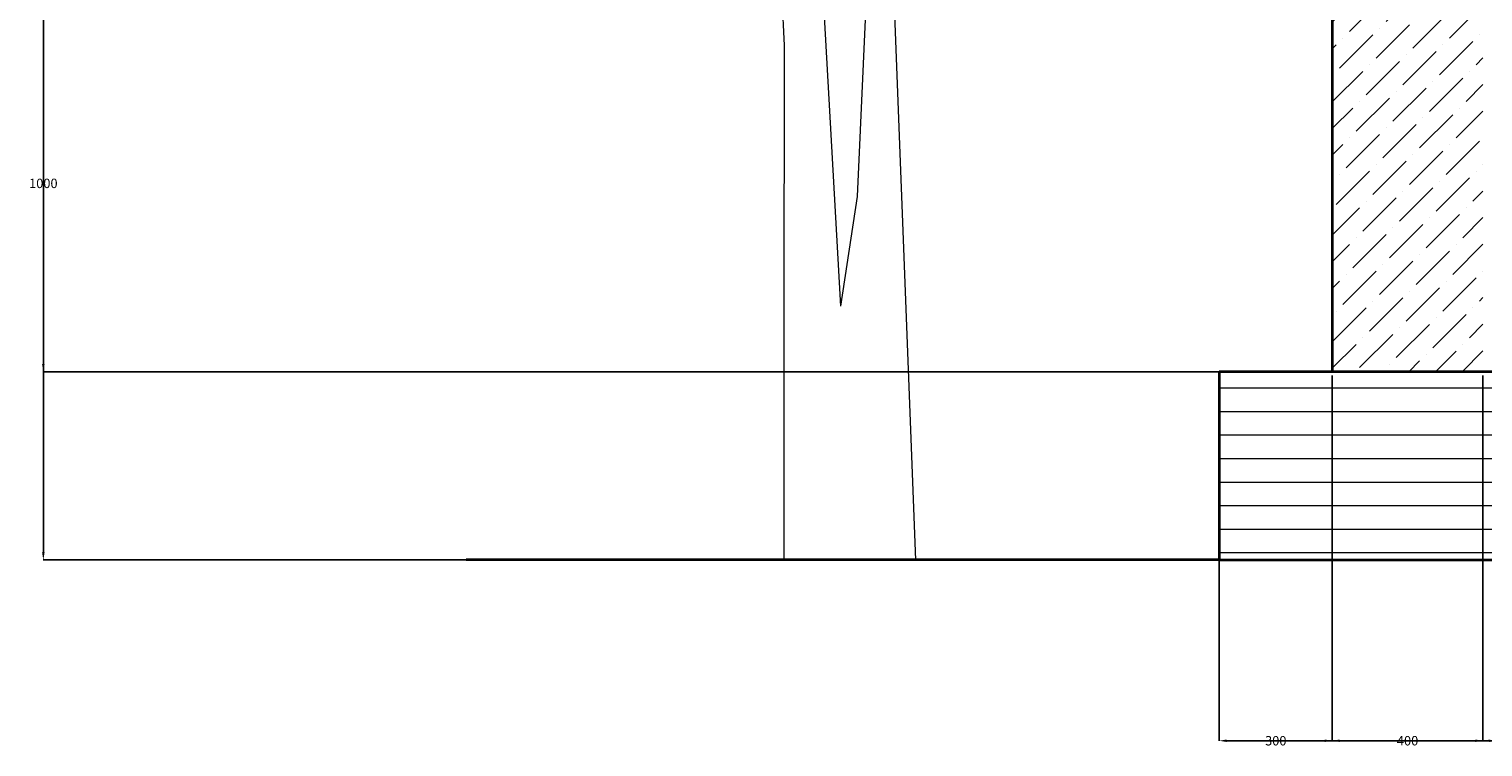
# Model space of a CAD drawing. Units: millimetres. Extents: x -692 to 9639, y -141 to 10345.
# Tile 1 of 19: x -687 to 3174, y -141 to 1765. Entities that reach past the tile are written whole.
import ezdxf

# ---------------------------------------------------------------- set-up
doc = ezdxf.new("R2010")
doc.units = ezdxf.units.MM
doc.header["$MEASUREMENT"] = 0
for name, color, linetype, lineweight in [('A-ANNO-DIMS', 2, 'Continuous', 18), ('A-ELEV', 7, 'Continuous', 35), ('A-ELEV-PATT', 8, 'Continuous', 13), ('L-PLNT', 3, 'Continuous', 18)]:
    doc.layers.add(name, color=color, linetype=linetype, lineweight=lineweight)
doc.styles.get("Standard").update_dxf_attribs({"font": 'arial.ttf'})
doc.dimstyles.get("Standard").update_dxf_attribs({"dimtxt": 25, "dimasz": 20, "dimexe": 0.18, "dimexo": 10, "dimgap": 10, "dimtad": 0, "dimtih": 1, "dimtoh": 1, "dimdec": 0, "dimzin": 0, "dimdsep": 46, "dimtxsty": 'Standard', "dimcen": 10, "dimadec": 0, "dimazin": 0, "dimtfac": 1, "dimtdec": 0, "dimtofl": 0, "dimtmove": 0, "dimatfit": 3, "dimfxl": 1, "dimtolj": 1, "dimtzin": 0, "dimarcsym": 0})

# ---------------------------------------------------------------- blocks, each defined once
blk = doc.blocks.new('*D6')
at = {"layer": 'A-ANNO-DIMS', "color": 0, "lineweight": -2, "transparency": 16777216}
for p, q in [((2473.7, 345.6), (2473.7, -124.6)), ((9073.7, 345.6), (9073.7, -124.6)), ((2493.7, -124.4), (5726.4, -124.4)), ((9053.7, -124.4), (5821.1, -124.4))]:
    blk.add_line(p, q, dxfattribs=at)
at = {"layer": 'A-ANNO-DIMS', "color": 0, "lineweight": -3, "transparency": 16777216}
for points in [[(2493.7, -121.1), (2493.7, -127.8), (2473.7, -124.4)], [(9053.7, -121.1), (9053.7, -127.8), (9073.7, -124.4)]]:
    blk.add_solid(points, dxfattribs=at)
at = {"layer": 'Defpoints', "color": 0, "lineweight": -3, "transparency": 16777216}
for p in [(2473.7, 355.6), (9073.7, 355.6), (9073.7, -124.4)]:
    blk.add_point(p, dxfattribs=at)
at = {"layer": 'A-ANNO-DIMS', "color": 0, "transparency": 16777216, "insert": (5773.7, -124.4), "char_height": 25, "attachment_point": 5}
blk.add_mtext('\\A1;6600', dxfattribs=at)
blk = doc.blocks.new('*D7')
at = {"layer": 'A-ANNO-DIMS', "color": 0, "lineweight": -2, "transparency": 16777216}
for p, q in [((8481.5, 9848.8), (-649.1, 9848.8)), ((-648.9, 9828.8), (-648.9, 5124.9)), ((-648.9, 375.6), (-648.9, 5079.4)), ((2463.7, 355.6), (-649.1, 355.6))]:
    blk.add_line(p, q, dxfattribs=at)
at = {"layer": 'A-ANNO-DIMS', "color": 0, "lineweight": -3, "transparency": 16777216}
for points in [[(-652.2, 9828.8), (-645.6, 9828.8), (-648.9, 9848.8)], [(-652.2, 375.6), (-645.6, 375.6), (-648.9, 355.6)]]:
    blk.add_solid(points, dxfattribs=at)
at = {"layer": 'Defpoints', "color": 0, "lineweight": -3, "transparency": 16777216}
for p in [(-648.9, 9848.8), (8491.5, 9848.8), (2473.7, 355.6)]:
    blk.add_point(p, dxfattribs=at)
at = {"layer": 'A-ANNO-DIMS', "color": 0, "transparency": 16777216, "insert": (-648.9, 5102.2), "char_height": 25, "attachment_point": 5}
blk.add_mtext('\\A1;9493', dxfattribs=at)
blk = doc.blocks.new('*D18')
at = {"layer": 'A-ANNO-DIMS', "color": 0, "lineweight": -2, "transparency": 16777216}
for p, q in [((2473.7, 845.6), (2473.7, -124.6)), ((2773.7, 845.6), (2773.7, -124.6)), ((2493.7, -124.4), (2586.2, -124.4)), ((2753.7, -124.4), (2661.3, -124.4))]:
    blk.add_line(p, q, dxfattribs=at)
at = {"layer": 'A-ANNO-DIMS', "color": 0, "lineweight": -3, "transparency": 16777216}
for points in [[(2493.7, -121.1), (2493.7, -127.8), (2473.7, -124.4)], [(2753.7, -121.1), (2753.7, -127.8), (2773.7, -124.4)]]:
    blk.add_solid(points, dxfattribs=at)
at = {"layer": 'Defpoints', "color": 0, "lineweight": -3, "transparency": 16777216}
for p in [(2473.7, 855.6), (2773.7, 855.6), (2773.7, -124.4)]:
    blk.add_point(p, dxfattribs=at)
at = {"layer": 'A-ANNO-DIMS', "color": 0, "transparency": 16777216, "insert": (2623.7, -124.4), "char_height": 25, "attachment_point": 5}
blk.add_mtext('\\A1;300', dxfattribs=at)
blk = doc.blocks.new('*D19')
at = {"layer": 'A-ANNO-DIMS', "color": 0, "lineweight": -2, "transparency": 16777216}
for p, q in [((2773.7, 845.6), (2773.7, -124.6)), ((3173.7, 845.6), (3173.7, -124.6)), ((2793.7, -124.4), (2935.7, -124.4)), ((3153.7, -124.4), (3011.8, -124.4))]:
    blk.add_line(p, q, dxfattribs=at)
at = {"layer": 'A-ANNO-DIMS', "color": 0, "lineweight": -3, "transparency": 16777216}
for points in [[(2793.7, -121.1), (2793.7, -127.8), (2773.7, -124.4)], [(3153.7, -121.1), (3153.7, -127.8), (3173.7, -124.4)]]:
    blk.add_solid(points, dxfattribs=at)
at = {"layer": 'Defpoints', "color": 0, "lineweight": -3, "transparency": 16777216}
for p in [(2773.7, 855.6), (3173.7, 855.6), (3173.7, -124.4)]:
    blk.add_point(p, dxfattribs=at)
at = {"layer": 'A-ANNO-DIMS', "color": 0, "transparency": 16777216, "insert": (2973.7, -124.4), "char_height": 25, "attachment_point": 5}
blk.add_mtext('\\A1;400', dxfattribs=at)
blk = doc.blocks.new('*D20')
at = {"layer": 'A-ANNO-DIMS', "color": 0, "lineweight": -2, "transparency": 16777216}
for p, q in [((3173.7, 845.6), (3173.7, -124.6)), ((5373.7, 845.6), (5373.7, -124.6)), ((3193.7, -124.4), (4226.2, -124.4)), ((5353.7, -124.4), (4321.2, -124.4))]:
    blk.add_line(p, q, dxfattribs=at)
at = {"layer": 'A-ANNO-DIMS', "color": 0, "lineweight": -3, "transparency": 16777216}
for points in [[(3193.7, -121.1), (3193.7, -127.8), (3173.7, -124.4)], [(5353.7, -121.1), (5353.7, -127.8), (5373.7, -124.4)]]:
    blk.add_solid(points, dxfattribs=at)
at = {"layer": 'Defpoints', "color": 0, "lineweight": -3, "transparency": 16777216}
for p in [(3173.7, 855.6), (5373.7, 855.6), (5373.7, -124.4)]:
    blk.add_point(p, dxfattribs=at)
at = {"layer": 'A-ANNO-DIMS', "color": 0, "transparency": 16777216, "insert": (4273.7, -124.4), "char_height": 25, "attachment_point": 5}
blk.add_mtext('\\A1;2200', dxfattribs=at)
blk = doc.blocks.new('*D25')
at = {"layer": 'A-ANNO-DIMS', "color": 0, "lineweight": -2, "transparency": 16777216}
for p, q in [((3163.7, 1855.6), (-649.1, 1855.6)), ((-648.9, 1835.6), (-648.9, 1378.3)), ((-648.9, 875.6), (-648.9, 1332.8)), ((2763.7, 855.6), (-649.1, 855.6))]:
    blk.add_line(p, q, dxfattribs=at)
at = {"layer": 'A-ANNO-DIMS', "color": 0, "lineweight": -3, "transparency": 16777216}
for points in [[(-652.2, 1835.6), (-645.6, 1835.6), (-648.9, 1855.6)], [(-652.2, 875.6), (-645.6, 875.6), (-648.9, 855.6)]]:
    blk.add_solid(points, dxfattribs=at)
at = {"layer": 'Defpoints', "color": 0, "lineweight": -3, "transparency": 16777216}
for p in [(-648.9, 1855.6), (3173.7, 1855.6), (2773.7, 855.6)]:
    blk.add_point(p, dxfattribs=at)
at = {"layer": 'A-ANNO-DIMS', "color": 0, "transparency": 16777216, "insert": (-648.9, 1355.6), "char_height": 25, "attachment_point": 5}
blk.add_mtext('\\A1;1000', dxfattribs=at)

msp = doc.modelspace()

# ---------------------------------------------------------------- hatches: boundary and pattern name
at = {"layer": 'A-ELEV-PATT'}
h = msp.add_hatch(dxfattribs=at)
h.set_pattern_fill('ANSI36', color=256, scale=400)
edge = h.paths.add_edge_path()
edge.add_spline(control_points=[(3173.746, 2309.965), (3085.901, 2332.226), (2969.139, 2424.713), (2876.436, 2493.45)], knot_values=[20955.88576955, 20955.88576955, 20955.88576955, 20955.88576955, 21219.85539585, 21219.85539585, 21219.85539585, 21219.85539585], degree=3, periodic=0)
edge.add_spline(control_points=[(2876.436, 2493.45), (2855.134, 2468.311), (2819.135, 2451.154), (2773.746, 2440.514)], knot_values=[5238.08213467, 5238.08213467, 5238.08213467, 5238.08213467, 5382.8513026, 5382.8513026, 5382.8513026, 5382.8513026], degree=3, periodic=0)
edge.add_line((2773.746, 2440.514), (2773.746, 2354.397))
edge.add_spline(control_points=[(2773.746, 2354.397), (2777.278, 2343.918), (2780.812, 2333.449), (2784.279, 2323.093)], knot_values=[20514.20511429, 20514.20511429, 20514.20511429, 20514.20511429, 20537.39604293, 20537.39604293, 20537.39604293, 20537.39604293], degree=3, periodic=0)
edge.add_spline(control_points=[(2784.279, 2323.093), (2849.257, 2305.468), (3007.384, 2255.171), (2928.441, 2185.016), (2819.76, 2148.371)], knot_values=[1896.27813718, 1896.27813718, 1896.27813718, 1896.27813718, 2077.70067144, 2424.51760392, 2424.51760392, 2424.51760392, 2424.51760392], degree=3, periodic=0)
edge.add_spline(control_points=[(2819.76, 2148.371), (2817.899, 2146.748), (2815.52, 2145.926), (2812.57, 2145.987)], knot_values=[20304.87329269, 20304.87329269, 20304.87329269, 20304.87329269, 20326.21847821, 20326.21847821, 20326.21847821, 20326.21847821], degree=3, periodic=0)
edge.add_spline(control_points=[(2812.57, 2145.987), (2800.291, 2141.985), (2787.329, 2138.102), (2773.746, 2134.363)], knot_values=[1850.39591646, 1850.39591646, 1850.39591646, 1850.39591646, 1888.716341, 1888.716341, 1888.716341, 1888.716341], degree=3, periodic=0)
edge.add_line((2773.746, 2134.363), (2773.746, 855.575))
edge.add_line((2773.746, 855.575), (3173.746, 855.575))
edge.add_line((3173.746, 855.575), (3173.746, 2309.965))
edge = h.paths.add_edge_path()
edge.add_spline(control_points=[(3420.651, 2717.101), (3368.378, 2761.363), (3299.425, 2803.396), (3225.3, 2834.508)], knot_values=[12552.99587302, 12552.99587302, 12552.99587302, 12552.99587302, 12712.02358035, 12712.02358035, 12712.02358035, 12712.02358035], degree=3, periodic=0)
edge.add_spline(control_points=[(3225.3, 2834.508), (3218.267, 2754.576), (3174.644, 2682.922), (3107.112, 2626.403)], knot_values=[8572.46293399, 8572.46293399, 8572.46293399, 8572.46293399, 8814.86919927, 8814.86919927, 8814.86919927, 8814.86919927], degree=3, periodic=0)
edge.add_spline(control_points=[(3107.112, 2626.403), (3129.755, 2627.593), (3152.034, 2628.996), (3173.746, 2630.586)], knot_values=[10558.19039557, 10558.19039557, 10558.19039557, 10558.19039557, 10599.03834951, 10599.03834951, 10599.03834951, 10599.03834951], degree=3, periodic=0)
edge.add_line((3173.746, 2630.586), (3173.746, 2648.27))
edge.add_line((3173.746, 2648.27), (3219.774, 2648.27))
edge.add_spline(control_points=[(3219.774, 2648.27), (3215.509, 2669.279), (3223.352, 2735.229), (3357.845, 2728.872), (3420.651, 2717.101)], knot_values=[11042.13010686, 11042.13010686, 11042.13010686, 11042.13010686, 11110.4948836, 11298.41454305, 11298.41454305, 11298.41454305, 11298.41454305], degree=3, periodic=0)
edge = h.paths.add_edge_path()
edge.add_spline(control_points=[(3107.112, 2626.403), (3174.644, 2682.922), (3218.267, 2754.576), (3225.3, 2834.508)], knot_values=[8572.46293399, 8572.46293399, 8572.46293399, 8572.46293399, 8814.86919927, 8814.86919927, 8814.86919927, 8814.86919927], degree=3, periodic=0)
edge.add_spline(control_points=[(3225.3, 2834.508), (3213.709, 2839.374), (3201.991, 2843.972), (3190.19, 2848.27)], knot_values=[12712.02358035, 12712.02358035, 12712.02358035, 12712.02358035, 12736.8923557, 12736.8923557, 12736.8923557, 12736.8923557], degree=3, periodic=0)
edge.add_line((3190.19, 2848.27), (2928.387, 2848.27))
edge.add_spline(control_points=[(2928.387, 2848.27), (2886.081, 2816.098), (2840.884, 2784.767), (2798.089, 2758.256)], knot_values=[14939.29716066, 14939.29716066, 14939.29716066, 14939.29716066, 15046.25935392, 15046.25935392, 15046.25935392, 15046.25935392], degree=3, periodic=0)
edge.add_spline(control_points=[(2798.089, 2758.256), (2836.427, 2711.897), (2866.292, 2664.879), (2883.022, 2622.327)], knot_values=[5561.23366662, 5561.23366662, 5561.23366662, 5561.23366662, 5704.57044689, 5704.57044689, 5704.57044689, 5704.57044689], degree=3, periodic=0)
edge.add_spline(control_points=[(2883.022, 2622.327), (2956.927, 2620.92), (3033.919, 2622.554), (3107.112, 2626.403)], knot_values=[10426.14846168, 10426.14846168, 10426.14846168, 10426.14846168, 10558.19039557, 10558.19039557, 10558.19039557, 10558.19039557], degree=3, periodic=0)
edge = h.paths.add_edge_path()
edge.add_spline(control_points=[(3173.746, 2630.586), (3152.034, 2628.996), (3129.755, 2627.593), (3107.112, 2626.403)], knot_values=[10558.19039557, 10558.19039557, 10558.19039557, 10558.19039557, 10599.03834951, 10599.03834951, 10599.03834951, 10599.03834951], degree=3, periodic=0)
edge.add_spline(control_points=[(3107.112, 2626.403), (3049.969, 2578.578), (2975.708, 2541.59), (2892.012, 2519.592)], knot_values=[8367.34849038, 8367.34849038, 8367.34849038, 8367.34849038, 8572.46293399, 8572.46293399, 8572.46293399, 8572.46293399], degree=3, periodic=0)
edge.add_spline(control_points=[(2892.012, 2519.592), (2888.384, 2510.058), (2883.137, 2501.359), (2876.436, 2493.45)], knot_values=[5382.8513026, 5382.8513026, 5382.8513026, 5382.8513026, 5428.39625745, 5428.39625745, 5428.39625745, 5428.39625745], degree=3, periodic=0)
edge.add_spline(control_points=[(2876.436, 2493.45), (2969.139, 2424.713), (3085.901, 2332.226), (3173.746, 2309.965)], knot_values=[20955.88576955, 20955.88576955, 20955.88576955, 20955.88576955, 21219.85539585, 21219.85539585, 21219.85539585, 21219.85539585], degree=3, periodic=0)
edge.add_line((3173.746, 2309.965), (3173.746, 2630.586))
edge = h.paths.add_edge_path(flags=17)
edge.add_spline(control_points=[(2819.76, 2148.371), (2928.441, 2185.016), (3007.384, 2255.171), (2849.257, 2305.468), (2784.279, 2323.093)], knot_values=[1896.27813718, 1896.27813718, 1896.27813718, 1896.27813718, 2243.09506965, 2424.51760392, 2424.51760392, 2424.51760392, 2424.51760392], degree=3, periodic=0)
edge.add_spline(control_points=[(2784.279, 2323.093), (2812.387, 2239.151), (2836.152, 2162.664), (2819.76, 2148.371)], knot_values=[20326.21847821, 20326.21847821, 20326.21847821, 20326.21847821, 20514.20511429, 20514.20511429, 20514.20511429, 20514.20511429], degree=3, periodic=0)
edge = h.paths.add_edge_path(flags=17)
edge.add_spline(control_points=[(2819.76, 2148.371), (2836.152, 2162.664), (2812.387, 2239.151), (2784.279, 2323.093)], knot_values=[20326.21847821, 20326.21847821, 20326.21847821, 20326.21847821, 20514.20511429, 20514.20511429, 20514.20511429, 20514.20511429], degree=3, periodic=0)
edge.add_spline(control_points=[(2784.279, 2323.093), (2780.798, 2324.038), (2777.286, 2324.983), (2773.746, 2325.93)], knot_values=[2424.51760392, 2424.51760392, 2424.51760392, 2424.51760392, 2434.23800618, 2434.23800618, 2434.23800618, 2434.23800618], degree=3, periodic=0)
edge.add_line((2773.746, 2325.93), (2773.746, 2166.486))
edge.add_spline(control_points=[(2773.746, 2166.486), (2790.303, 2153.967), (2803.9, 2146.166), (2812.57, 2145.987)], knot_values=[20242.12265912, 20242.12265912, 20242.12265912, 20242.12265912, 20304.87329269, 20304.87329269, 20304.87329269, 20304.87329269], degree=3, periodic=0)
edge.add_spline(control_points=[(2812.57, 2145.987), (2814.994, 2146.777), (2817.39, 2147.572), (2819.76, 2148.371)], knot_values=[1888.716341, 1888.716341, 1888.716341, 1888.716341, 1896.27813718, 1896.27813718, 1896.27813718, 1896.27813718], degree=3, periodic=0)
edge = h.paths.add_edge_path()
edge.add_spline(control_points=[(2892.012, 2519.592), (2893.653, 2523.907), (2902.094, 2552.818), (2896.12, 2589.012), (2883.022, 2622.327)], knot_values=[5428.39625745, 5428.39625745, 5428.39625745, 5428.39625745, 5449.01011401, 5561.23366662, 5561.23366662, 5561.23366662, 5561.23366662], degree=3, periodic=0)
edge.add_spline(control_points=[(2883.022, 2622.327), (2845.501, 2623.042), (2808.775, 2624.54), (2773.746, 2626.93)], knot_values=[10359.11175247, 10359.11175247, 10359.11175247, 10359.11175247, 10426.14846168, 10426.14846168, 10426.14846168, 10426.14846168], degree=3, periodic=0)
edge.add_line((2773.746, 2626.93), (2773.746, 2561.8))
edge.add_spline(control_points=[(2773.746, 2561.8), (2795.257, 2551.206), (2822.448, 2532.82), (2853.096, 2510.59)], knot_values=[20841.44589883, 20841.44589883, 20841.44589883, 20841.44589883, 20933.19502211, 20933.19502211, 20933.19502211, 20933.19502211], degree=3, periodic=0)
edge.add_spline(control_points=[(2853.096, 2510.59), (2866.269, 2513.232), (2879.25, 2516.238), (2892.012, 2519.592)], knot_values=[8336.07392909, 8336.07392909, 8336.07392909, 8336.07392909, 8367.34849038, 8367.34849038, 8367.34849038, 8367.34849038], degree=3, periodic=0)
edge = h.paths.add_edge_path(flags=17)
edge.add_spline(control_points=[(2892.012, 2519.592), (2975.708, 2541.59), (3049.969, 2578.578), (3107.112, 2626.403)], knot_values=[8367.34849038, 8367.34849038, 8367.34849038, 8367.34849038, 8572.46293399, 8572.46293399, 8572.46293399, 8572.46293399], degree=3, periodic=0)
edge.add_spline(control_points=[(3107.112, 2626.403), (3033.919, 2622.554), (2956.927, 2620.92), (2883.022, 2622.327)], knot_values=[10426.14846168, 10426.14846168, 10426.14846168, 10426.14846168, 10558.19039557, 10558.19039557, 10558.19039557, 10558.19039557], degree=3, periodic=0)
edge.add_spline(control_points=[(2883.022, 2622.327), (2896.12, 2589.012), (2902.094, 2552.818), (2893.653, 2523.907), (2892.012, 2519.592)], knot_values=[5428.39625745, 5428.39625745, 5428.39625745, 5428.39625745, 5540.61981006, 5561.23366662, 5561.23366662, 5561.23366662, 5561.23366662], degree=3, periodic=0)
edge = h.paths.add_edge_path()
edge.add_spline(control_points=[(2773.746, 2440.514), (2819.135, 2451.154), (2855.134, 2468.311), (2876.436, 2493.45)], knot_values=[5238.08213467, 5238.08213467, 5238.08213467, 5238.08213467, 5382.8513026, 5382.8513026, 5382.8513026, 5382.8513026], degree=3, periodic=0)
edge.add_spline(control_points=[(2876.436, 2493.45), (2868.467, 2499.359), (2860.676, 2505.092), (2853.096, 2510.59)], knot_values=[20933.19502211, 20933.19502211, 20933.19502211, 20933.19502211, 20955.88576955, 20955.88576955, 20955.88576955, 20955.88576955], degree=3, periodic=0)
edge.add_spline(control_points=[(2853.096, 2510.59), (2827.314, 2505.418), (2800.796, 2501.637), (2773.746, 2499.359)], knot_values=[8274.86392127, 8274.86392127, 8274.86392127, 8274.86392127, 8336.07392909, 8336.07392909, 8336.07392909, 8336.07392909], degree=3, periodic=0)
edge.add_line((2773.746, 2499.359), (2773.746, 2440.514))
edge = h.paths.add_edge_path()
edge.add_spline(control_points=[(2883.022, 2622.327), (2866.292, 2664.879), (2836.427, 2711.897), (2798.089, 2758.256)], knot_values=[5561.23366662, 5561.23366662, 5561.23366662, 5561.23366662, 5704.57044689, 5704.57044689, 5704.57044689, 5704.57044689], degree=3, periodic=0)
edge.add_spline(control_points=[(2798.089, 2758.256), (2789.874, 2753.166), (2781.747, 2748.254), (2773.746, 2743.548)], knot_values=[15046.25935392, 15046.25935392, 15046.25935392, 15046.25935392, 15066.79294618, 15066.79294618, 15066.79294618, 15066.79294618], degree=3, periodic=0)
edge.add_line((2773.746, 2743.548), (2773.746, 2626.93))
edge.add_spline(control_points=[(2773.746, 2626.93), (2808.775, 2624.54), (2845.501, 2623.042), (2883.022, 2622.327)], knot_values=[10359.11175247, 10359.11175247, 10359.11175247, 10359.11175247, 10426.14846168, 10426.14846168, 10426.14846168, 10426.14846168], degree=3, periodic=0)
edge = h.paths.add_edge_path()
edge.add_spline(control_points=[(2798.089, 2758.256), (2840.884, 2784.767), (2886.081, 2816.098), (2928.387, 2848.27)], knot_values=[14939.29716066, 14939.29716066, 14939.29716066, 14939.29716066, 15046.25935392, 15046.25935392, 15046.25935392, 15046.25935392], degree=3, periodic=0)
edge.add_line((2928.387, 2848.27), (2773.746, 2848.27))
edge.add_line((2773.746, 2848.27), (2773.746, 2786.349))
edge.add_spline(control_points=[(2773.746, 2786.349), (2782.183, 2777.04), (2790.311, 2767.662), (2798.089, 2758.256)], knot_values=[5704.57044689, 5704.57044689, 5704.57044689, 5704.57044689, 5733.65273084, 5733.65273084, 5733.65273084, 5733.65273084], degree=3, periodic=0)
edge = h.paths.add_edge_path()
edge.add_spline(control_points=[(3463.702, 2676.006), (3451.141, 2689.747), (3436.681, 2703.529), (3420.651, 2717.101)], knot_values=[12504.23047843, 12504.23047843, 12504.23047843, 12504.23047843, 12552.99587302, 12552.99587302, 12552.99587302, 12552.99587302], degree=3, periodic=0)
edge.add_spline(control_points=[(3420.651, 2717.101), (3357.845, 2728.872), (3223.352, 2735.229), (3215.509, 2669.279), (3219.774, 2648.27)], knot_values=[11042.13010686, 11042.13010686, 11042.13010686, 11042.13010686, 11230.04976631, 11298.41454305, 11298.41454305, 11298.41454305, 11298.41454305], degree=3, periodic=0)
edge.add_line((3219.774, 2648.27), (3341.426, 2648.27))
edge.add_spline(control_points=[(3341.426, 2648.27), (3397.595, 2656.506), (3440.895, 2666.057), (3463.702, 2676.006)], knot_values=[10715.9300286, 10715.9300286, 10715.9300286, 10715.9300286, 10852.53626518, 10852.53626518, 10852.53626518, 10852.53626518], degree=3, periodic=0)
edge = h.paths.add_edge_path()
edge.add_spline(control_points=[(2853.096, 2510.59), (2822.448, 2532.82), (2795.257, 2551.206), (2773.746, 2561.8)], knot_values=[20841.44589883, 20841.44589883, 20841.44589883, 20841.44589883, 20933.19502211, 20933.19502211, 20933.19502211, 20933.19502211], degree=3, periodic=0)
edge.add_line((2773.746, 2561.8), (2773.746, 2499.359))
edge.add_spline(control_points=[(2773.746, 2499.359), (2800.796, 2501.637), (2827.314, 2505.418), (2853.096, 2510.59)], knot_values=[8274.86392127, 8274.86392127, 8274.86392127, 8274.86392127, 8336.07392909, 8336.07392909, 8336.07392909, 8336.07392909], degree=3, periodic=0)
h = msp.add_hatch(dxfattribs=at)
h.set_pattern_fill('LINE', color=256, scale=500)
h.paths.add_polyline_path([(9073.746, 855.575), (8773.746, 855.575), (7273.746, 855.575), (2773.746, 855.575), (2473.746, 855.575), (2473.746, 355.575), (9073.746, 355.575)])

# ---------------------------------------------------------------- linework, layer by layer
at = {"layer": 'A-ELEV'}
for p, q in [((2773.746, 2848.27), (2773.746, 855.575)), ((2773.746, 855.575), (2473.746, 855.575)), ((2473.746, 855.575), (2473.746, 355.575)), ((7273.746, 855.575), (2773.746, 855.575)), ((2473.746, 355.575), (473.746, 355.575)), ((2473.746, 355.575), (9073.746, 355.575))]:
    msp.add_line(p, q, dxfattribs=at)
at = {"layer": 'L-PLNT'}
for p, q in [((1301.056, 2077.694), (1317.991, 1721.29)), ((1512.588, 1320.381), (1543.202, 1990.116)), ((1668.259, 355.575), (1608.333, 1905.92)), ((1468.429, 1029.289), (1424.921, 1814.529)), ((1317.991, 1721.29), (1317.707, 987.833)), ((1468.429, 1029.289), (1512.588, 1320.381)), ((1317.707, 987.833), (1317.462, 355.575))]:
    msp.add_line(p, q, dxfattribs=at)

# ---------------------------------------------------------------- dimensions: what is measured, and where the dimension line sits
at = {"layer": 'A-ANNO-DIMS'}
for base, p1, p2, picture, middle in [((-648.912, 9848.772), (2473.746, 355.575), (8491.547, 9848.772), '*D7', (-648.912, 5102.173)), ((-648.912, 1855.575), (2773.746, 855.575), (3173.746, 1855.575), '*D25', (-648.912, 1355.575))]:
    dim = msp.add_linear_dim(base=base, p1=p1, p2=p2, angle=90, dimstyle='Standard', override={"dimdec": 0, "dimlfac": 1, "dimrnd": 0, "dimzin": 0, "dimdsep": 46, "dimlunit": 2}, dxfattribs=at)
    dim.commit()
    dim.dimension.update_dxf_attribs({"geometry": picture, "text_midpoint": middle})
for base, p1, p2, picture, middle in [((2773.746, -124.425), (2473.746, 855.575), (2773.746, 855.575), '*D18', (2623.746, -124.425)), ((3173.746, -124.425), (2773.746, 855.575), (3173.746, 855.575), '*D19', (2973.746, -124.425)), ((5373.746, -124.425), (3173.746, 855.575), (5373.746, 855.575), '*D20', (4273.746, -124.425)), ((9073.746, -124.425), (2473.746, 355.575), (9073.746, 355.575), '*D6', (5773.746, -124.425))]:
    dim = msp.add_linear_dim(base=base, p1=p1, p2=p2, dimstyle='Standard', override={"dimdec": 0, "dimlfac": 1, "dimrnd": 0, "dimzin": 0, "dimdsep": 46, "dimlunit": 2}, dxfattribs=at)
    dim.commit()
    dim.dimension.update_dxf_attribs({"geometry": picture, "text_midpoint": middle})

doc.saveas('drawing.dxf')
